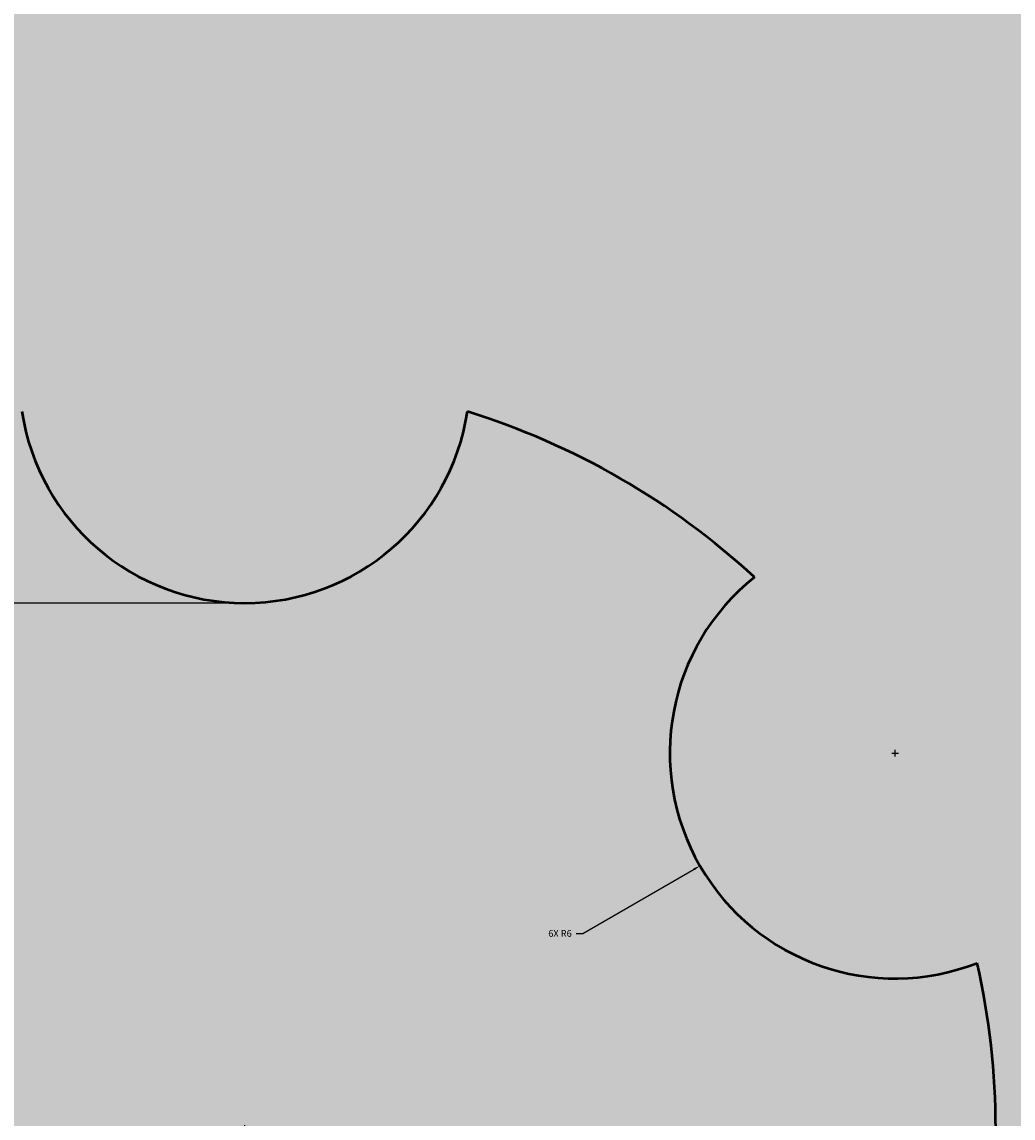
# Model space of a CAD drawing. Units: inches. Extents: x -13 to 107, y -48 to 102.
# Tile 8 of 13: x 22 to 48, y 14 to 43. Entities that reach past the tile are written whole.
import ezdxf

# ---------------------------------------------------------------- set-up
doc = ezdxf.new("R2010")
doc.units = ezdxf.units.IN
doc.header["$MEASUREMENT"] = 0
for name, color, linetype, lineweight in [('M-DIMS', 2, 'Continuous', 18), ('M-HATC', 8, 'Continuous', 18), ('M-OUTL', 7, 'Continuous', 50)]:
    doc.layers.add(name, color=color, linetype=linetype, lineweight=lineweight)
doc.styles.get("Standard").update_dxf_attribs({"font": 'arial.ttf'})
doc.dimstyles.get("Standard").update_dxf_attribs({"dimtxt": 0.18, "dimasz": 0.18, "dimexe": 0.18, "dimexo": 0.0625, "dimgap": 0.09, "dimtad": 0, "dimtih": 1, "dimtoh": 1, "dimdec": 4, "dimzin": 0, "dimdsep": 46, "dimtxsty": 'Standard', "dimcen": 0.09, "dimadec": 0, "dimazin": 0, "dimtfac": 1, "dimtdec": 4, "dimtofl": 0, "dimtmove": 0, "dimatfit": 3, "dimfxl": 1, "dimtolj": 1, "dimtzin": 0, "dimarcsym": 0})

# ---------------------------------------------------------------- blocks, each defined once
blk = doc.blocks.new('*D1')
at = {"layer": 'Defpoints', "color": 0, "transparency": 16777216}
for p in [(60.544, 101.543), (-5.45, 13.883), (60.544, 13.883)]:
    blk.add_point(p, dxfattribs=at)
at = {"layer": 'M-DIMS', "color": 0, "lineweight": -2, "transparency": 16777216}
for p, q in [((-5.45, 13.945), (-5.45, 101.723)), ((60.544, 13.945), (60.544, 101.723)), ((-5.27, 101.543), (27.328, 101.543)), ((60.364, 101.543), (27.766, 101.543))]:
    blk.add_line(p, q, dxfattribs=at)
at = {"layer": 'M-DIMS', "color": 0, "transparency": 16777216}
for points in [[(-5.27, 101.573), (-5.27, 101.513), (-5.45, 101.543)], [(60.364, 101.573), (60.364, 101.513), (60.544, 101.543)]]:
    blk.add_solid(points, dxfattribs=at)
at = {"layer": 'M-DIMS', "color": 0, "transparency": 16777216, "insert": (27.547, 101.543), "char_height": 0.18, "attachment_point": 5}
blk.add_mtext('\\A1;66', dxfattribs=at)
blk = doc.blocks.new('*D2')
at = {"layer": 'Defpoints', "color": 0, "transparency": 16777216}
for p in [(-12.585, 94.408), (27.547, 94.408), (27.547, -46.592)]:
    blk.add_point(p, dxfattribs=at)
at = {"layer": 'M-DIMS', "color": 0, "lineweight": -2, "transparency": 16777216}
for p, q in [((27.484, 94.408), (-12.765, 94.408)), ((-12.585, 94.228), (-12.585, 24.088)), ((-12.585, -46.412), (-12.585, 23.727)), ((27.484, -46.592), (-12.765, -46.592))]:
    blk.add_line(p, q, dxfattribs=at)
at = {"layer": 'M-DIMS', "color": 0, "transparency": 16777216}
for points in [[(-12.615, 94.228), (-12.555, 94.228), (-12.585, 94.408)], [(-12.615, -46.412), (-12.555, -46.412), (-12.585, -46.592)]]:
    blk.add_solid(points, dxfattribs=at)
at = {"layer": 'M-DIMS', "color": 0, "transparency": 16777216, "insert": (-12.585, 23.908), "char_height": 0.18, "attachment_point": 5}
blk.add_mtext('\\A1;141', dxfattribs=at)
blk = doc.blocks.new('*D4')
at = {"layer": 'Defpoints', "color": 0, "transparency": 16777216}
for p in [(27.547, 78.408), (67.679, 78.408), (27.547, 13.408)]:
    blk.add_point(p, dxfattribs=at)
at = {"layer": 'M-DIMS', "color": 0, "lineweight": -2, "transparency": 16777216}
for p, q in [((27.609, 78.408), (67.859, 78.408)), ((67.679, 78.228), (67.679, 46.09)), ((67.679, 13.588), (67.679, 45.726)), ((27.609, 13.408), (67.859, 13.408))]:
    blk.add_line(p, q, dxfattribs=at)
at = {"layer": 'M-DIMS', "color": 0, "transparency": 16777216}
for points in [[(67.649, 78.228), (67.709, 78.228), (67.679, 78.408)], [(67.649, 13.588), (67.709, 13.588), (67.679, 13.408)]]:
    blk.add_solid(points, dxfattribs=at)
at = {"layer": 'M-DIMS', "color": 0, "transparency": 16777216, "insert": (67.679, 45.908), "char_height": 0.18, "attachment_point": 5}
blk.add_mtext('\\A1;65', dxfattribs=at)
blk = doc.blocks.new('*D5')
at = {"layer": 'Defpoints', "color": 0, "transparency": 16777216}
for p in [(20.412, 27.408), (27.547, 27.408), (27.547, -0.592)]:
    blk.add_point(p, dxfattribs=at)
at = {"layer": 'M-DIMS', "color": 0, "lineweight": -2, "transparency": 16777216}
for p, q in [((27.484, 27.408), (20.232, 27.408)), ((20.412, 27.228), (20.412, 13.59)), ((20.412, -0.412), (20.412, 13.226)), ((27.484, -0.592), (20.232, -0.592))]:
    blk.add_line(p, q, dxfattribs=at)
at = {"layer": 'M-DIMS', "color": 0, "transparency": 16777216}
for points in [[(20.382, 27.228), (20.442, 27.228), (20.412, 27.408)], [(20.382, -0.412), (20.442, -0.412), (20.412, -0.592)]]:
    blk.add_solid(points, dxfattribs=at)
at = {"layer": 'M-DIMS', "color": 0, "transparency": 16777216, "insert": (20.412, 13.408), "char_height": 0.18, "attachment_point": 5}
blk.add_mtext('\\A1;28', dxfattribs=at)
blk = doc.blocks.new('*D9')
at = {"layer": 'Defpoints', "color": 0, "transparency": 16777216}
for p in [(17.547, 30.728), (27.547, 13.408)]:
    blk.add_point(p, dxfattribs=at)
at = {"layer": 'M-DIMS', "color": 0, "lineweight": -2, "transparency": 16777216}
for p, q in [((11.367, 41.121), (11.547, 41.121)), ((11.547, 41.121), (17.457, 30.884)), ((27.547, 13.318), (27.547, 13.498)), ((27.457, 13.408), (27.637, 13.408))]:
    blk.add_line(p, q, dxfattribs=at)
at = {"layer": 'M-DIMS', "color": 0, "transparency": 16777216}
blk.add_solid([(17.483, 30.899), (17.431, 30.869), (17.547, 30.728)], dxfattribs=at)
at = {"layer": 'M-DIMS', "color": 0, "transparency": 16777216, "insert": (10.868, 41.121), "char_height": 0.18, "attachment_point": 5}
blk.add_mtext('\\A1;6X R20', dxfattribs=at)
blk = doc.blocks.new('*D10')
at = {"layer": 'Defpoints', "color": 0, "transparency": 16777216}
for p in [(44.867, 23.408), (39.671, 20.408)]:
    blk.add_point(p, dxfattribs=at)
at = {"layer": 'M-DIMS', "color": 0, "lineweight": -2, "transparency": 16777216}
for p, q in [((44.777, 23.408), (44.957, 23.408)), ((44.867, 23.318), (44.867, 23.498)), ((36.553, 18.608), (39.515, 20.318)), ((36.373, 18.608), (36.553, 18.608))]:
    blk.add_line(p, q, dxfattribs=at)
at = {"layer": 'M-DIMS', "color": 0, "transparency": 16777216}
blk.add_solid([(39.5, 20.344), (39.53, 20.292), (39.671, 20.408)], dxfattribs=at)
at = {"layer": 'M-DIMS', "color": 0, "transparency": 16777216, "insert": (35.944, 18.608), "char_height": 0.18, "attachment_point": 5}
blk.add_mtext('\\A1;6X R6', dxfattribs=at)

msp = doc.modelspace()

# ---------------------------------------------------------------- hatches: boundary and pattern name
at = {"layer": 'M-HATC'}
h = msp.add_hatch(color=256, dxfattribs=at)
h.set_gradient(color1=(88, 186, 72), color2=(241, 235, 31), tint=1)
h.paths.add_polyline_path([(45.86, -14.044, 0.420873), (54.577, 32.339, -0.184081), (43.437, 76.537, 1.124637), (11.657, 76.537, -0.184081), (0.517, 32.339, 0.420873), (9.234, -14.044, -0.304084), (17.743, -34.622, 1.220926), (37.351, -34.622, -0.304084)])
h.paths.add_polyline_path([(33.479, -5.692, 0.859727), (21.615, -5.692, -0.111692), (13.972, -1.28, 0.859727), (8.04, 8.995, -0.111692), (8.04, 17.82, 0.859727), (13.972, 28.095, -0.111692), (21.615, 32.508, 0.859727), (33.479, 32.508, -0.111692), (41.122, 28.095, 0.859727), (47.054, 17.82, -0.111692), (47.054, 8.995, 0.859727), (41.122, -1.28, -0.111692)], flags=16)
h.paths.add_polyline_path([(32.547, -36.592, -1), (22.547, -36.592, -1)], flags=16)
h.paths.add_polyline_path([(17.547, 78.408, -1), (37.547, 78.408, -1)], flags=16)
h = msp.add_hatch(color=256, dxfattribs=at)
h.set_gradient(color1=(0, 0, 255), tint=1)
h.paths.add_polyline_path([(47.054, 8.995, 0.111692), (47.054, 17.82, -0.859727), (41.122, 28.095, 0.111692), (33.479, 32.508, -0.859727), (21.615, 32.508, 0.111692), (13.972, 28.095, -0.859727), (8.04, 17.82, 0.111692), (8.04, 8.995, -0.859727), (13.972, -1.28, 0.111692), (21.615, -5.692, -0.859727), (33.479, -5.692, 0.111692), (41.122, -1.28, -0.859727)])
h.paths.add_polyline_path([(37.547, 78.408, 1), (17.547, 78.408, 1)])
h.paths.add_polyline_path([(32.547, -36.592, 1), (22.547, -36.592, 1)])

# ---------------------------------------------------------------- linework, layer by layer
at = {"layer": 'M-OUTL'}
for centre, radius, start, end in [((106.998, 69.054), 64, 173.28544, 215.00666), ((27.547, 33.408), 6, 188.6269, 351.3731), ((27.547, 13.408), 20, 47.2539, 72.7461), ((27.547, 13.408), 33, 303.707, 35.0067), ((44.867, 23.408), 6, 128.6269, 291.3731), ((27.547, 13.408), 20, 347.2539, 12.7461)]:
    msp.add_arc(centre, radius, start, end, dxfattribs=at)

# ---------------------------------------------------------------- dimensions: what is measured, and where the dimension line sits
at = {"layer": 'M-DIMS'}
dim = msp.add_linear_dim(base=(60.544, 101.543), p1=(-5.45, 13.883), p2=(60.544, 13.883), dimstyle='Standard', override={"dimdec": 0, "dimlfac": 1, "dimrnd": 0, "dimzin": 0, "dimdsep": 46, "dimlunit": 2}, dxfattribs=at)
dim.commit()
dim.dimension.update_dxf_attribs({"geometry": '*D1', "text_midpoint": (27.547, 101.543)})
for base, p1, p2, picture, middle in [((-12.585, 94.408), (27.547, -46.592), (27.547, 94.408), '*D2', (-12.585, 23.908)), ((67.679, 78.408), (27.547, 13.408), (27.547, 78.408), '*D4', (67.679, 45.908)), ((20.412, 27.408), (27.547, -0.592), (27.547, 27.408), '*D5', (20.412, 13.408))]:
    dim = msp.add_linear_dim(base=base, p1=p1, p2=p2, angle=90, dimstyle='Standard', override={"dimdec": 0, "dimlfac": 1, "dimrnd": 0, "dimzin": 0, "dimdsep": 46, "dimlunit": 2}, dxfattribs=at)
    dim.commit()
    dim.dimension.update_dxf_attribs({"geometry": picture, "text_midpoint": middle})
for center, mpoint, picture, middle in [((27.547, 13.408), (17.547, 30.728), '*D9', (10.868, 41.121)), ((44.867, 23.408), (39.671, 20.408), '*D10', (35.944, 18.608))]:
    dim = msp.add_radius_dim(center=center, mpoint=mpoint, text='6X <>', dimstyle='Standard', override={"dimdec": 0, "dimlfac": 1, "dimrnd": 0, "dimzin": 0, "dimdsep": 46, "dimlunit": 2}, dxfattribs=at)
    dim.commit()
    dim.dimension.update_dxf_attribs({"geometry": picture, "text_midpoint": middle, "dimtype": 164})

doc.saveas('drawing.dxf')
